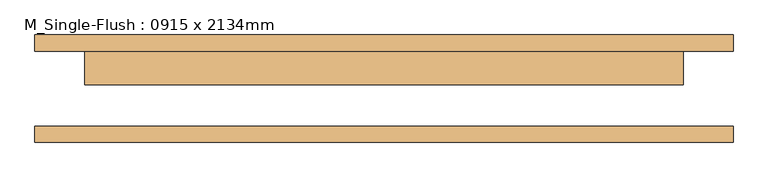
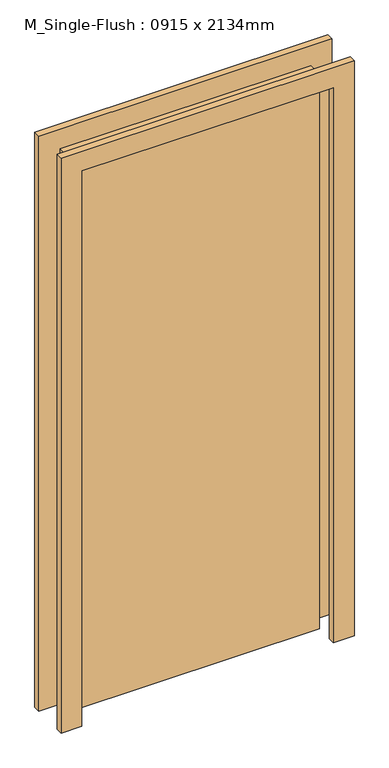
"""IFC4 building model written with IfcOpenShell, lengths in millimetres: door geometry, M_Single-Flush : 0915 x 2134mm."""

from ifc_helpers import new_model, si_unit, frame, origin, origin_with_axes, place, context, project, spatial, polyline, outline, extrude, source, transform, mapped, element, save


def m_single_flush_0915_x_2134mm_2427376d(model_context):
    return source(origin(), model_context, "Body", "SweptSolid", [
        extrude(outline(polyline([(2210.0, -533.5), (0.0, -533.5), (0.0, -457.5), (2134.0, -457.5), (2134.0, 457.5), (0.0, 457.5), (0.0, 533.5), (2210.0, 533.5), (2210.0, -533.5)])), frame((0.0, 57.15, 0.0), z_axis=(0.0, 1.0, 0.0), x_axis=(0.0, 0.0, 1.0)), (0.0, 0.0, 1.0), 25.0),
        extrude(outline(polyline([(2210.0, 533.5), (2210.0, -533.5), (0.0, -533.5), (0.0, -457.5), (2134.0, -457.5), (2134.0, 457.5), (0.0, 457.5), (0.0, 533.5), (2210.0, 533.5)])), frame((0.0, -82.15, 0.0), z_axis=(0.0, 1.0, 0.0), x_axis=(0.0, 0.0, 1.0)), (0.0, 0.0, 1.0), 25.0),
        extrude(outline(polyline([(457.5, 6.15), (-457.5, 6.15), (-457.5, 57.15), (457.5, 57.15), (457.5, 6.15)])), origin_with_axes(), (0.0, 0.0, 1.0), 2134.0),
    ])


if __name__ == "__main__":
    model = new_model("IFC4")
    model_context = context("Model", 3, world=origin())
    ifc_project = project(units=[si_unit("LENGTHUNIT", "METRE", prefix="MILLI")], contexts=[model_context])
    site = spatial("IfcSite", under=ifc_project)
    building = spatial("IfcBuilding", under=site)
    placement = place(None, origin())
    m_single_flush_0915_x_2134mm_shape = m_single_flush_0915_x_2134mm_2427376d(model_context)
    element("IfcDoor", 1, ObjectType="M_Single-Flush : 0915 x 2134mm", at=placement, inside=building, context=model_context, shape_type="MappedRepresentation", body=[
        mapped(m_single_flush_0915_x_2134mm_shape, transform((0.0, 0.0, 0.0), x_axis=(1.0, 0.0, 0.0), y_axis=(0.0, 1.0, 0.0), z_axis=(0.0, 0.0, 1.0))),
    ])
    save(model, "model.ifc")

# Revit data of these elements
# Type "M_Single-Flush : 0915 x 2134mm"
#   Type Mark = "15"
#   Thickness = 51 mm
#   Height = 2134 mm
#   Trim Projection Ext = 25 mm
#   Trim Projection Int = 25 mm
#   Trim Width = 76 mm
#   Width = 915 mm
#   Door Material = Door - Panel
#   Frame Material = Door - Frame
#   Function = (empty or 0)
#   Wall Closure = (empty or 0)
# Element 1 (IfcDoor, "M_Single-Flush : 0915 x 2134mm")
#   Materials on its faces: "Door - Frame", "Door - Panel"
# Materials
#   "Door - Panel": class "Wood", colour RGB 114 82 51, transparency 0
#   "Door - Frame": colour RGB 153 76 43, transparency 0
